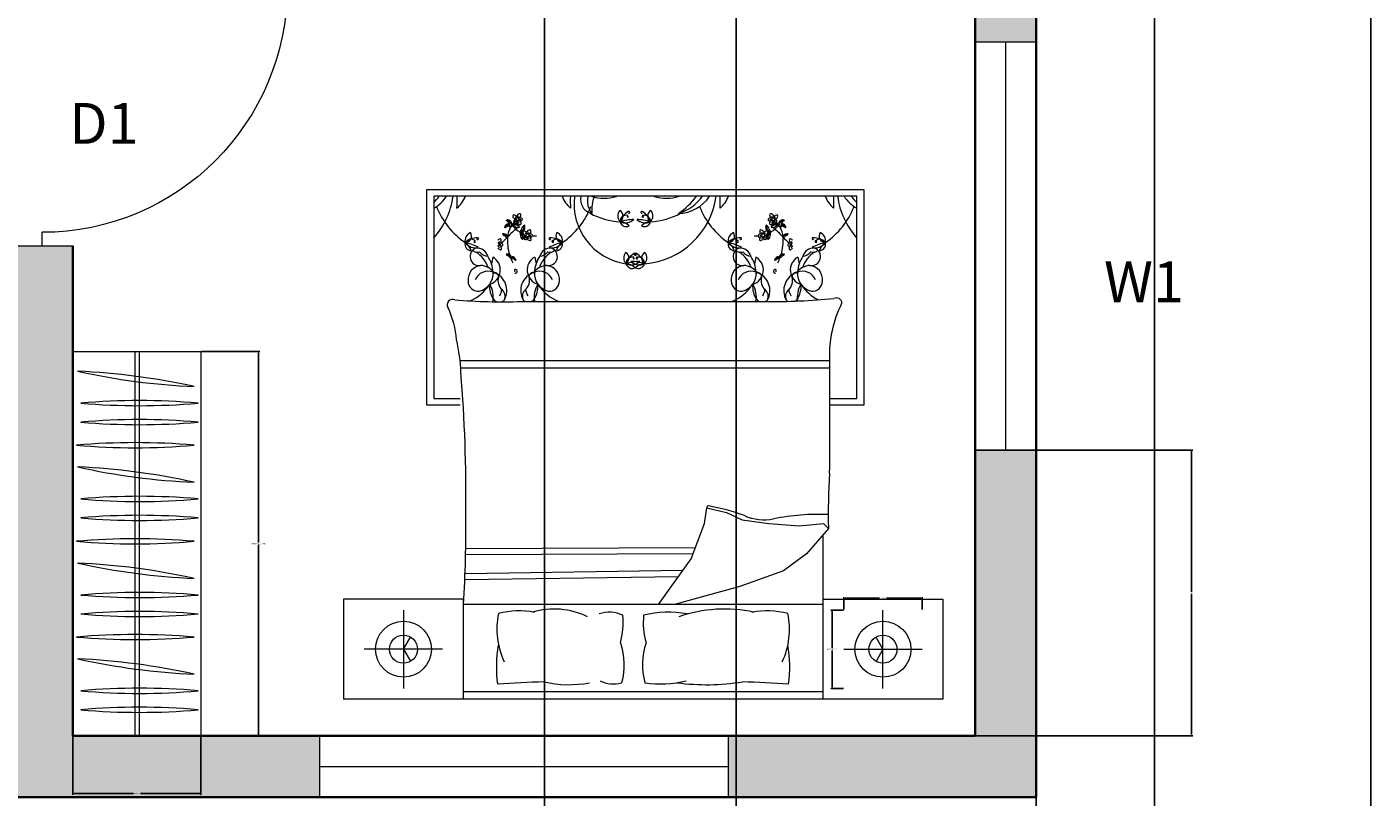
# Model space of a CAD drawing. Units: inches. Extents: x 5 to 421, y -617 to 43.
# Tile 8 of 15: x 223 to 421, y -465 to -351. Entities that reach past the tile are written whole.
import ezdxf

# ---------------------------------------------------------------- set-up
doc = ezdxf.new("R2010")
doc.units = ezdxf.units.IN
doc.header["$MEASUREMENT"] = 0
for name, color, linetype, lineweight in [('A-ANNO-DIMS', 2, 'Continuous', 18), ('A-ANNO-TEXT', 7, 'Continuous', 18), ('A-DOOR', 4, 'Continuous', 20), ('A-FLOR-CASE', 8, 'Continuous', 18), ('A-FURN', 8, 'Continuous', 13), ('A-GLAZ', 4, 'Continuous', 18), ('A-WALL', 7, 'Continuous', 35)]:
    doc.layers.add(name, color=color, linetype=linetype, lineweight=lineweight)
doc.layers.add('A-WALL-PATT', color=251, linetype='Continuous', lineweight=13, true_color=0x636466)
doc.styles.get("Standard").update_dxf_attribs({"font": 'arial.ttf'})
doc.dimstyles.get("Standard").update_dxf_attribs({"dimtxt": 0.18, "dimasz": 0.18, "dimexe": 0.18, "dimexo": 0.0625, "dimgap": 0.09, "dimtad": 0, "dimtih": 1, "dimtoh": 1, "dimdec": 0, "dimzin": 0, "dimdsep": 46, "dimlunit": 3, "dimtxsty": 'Standard', "dimcen": 0.09, "dimadec": 0, "dimazin": 0, "dimtfac": 1, "dimtdec": 0, "dimtofl": 0, "dimtmove": 0, "dimatfit": 3, "dimfxl": 1, "dimtolj": 1, "dimtzin": 0, "dimarcsym": 0})

# ---------------------------------------------------------------- blocks, each defined once
blk = doc.blocks.new('WINDOW-W1-60')
for p, q in [((0, 9), (60, 9)), ((0, 0), (0, 9)), ((60, 9), (60, 0)), ((0, 4.5), (60, 4.5)), ((60, 0), (0, 0))]:
    blk.add_line(p, q)
blk = doc.blocks.new('DOOR-SWING-36')
for p, q in [((35, 0), (35, 36)), ((36, 0), (36, 36))]:
    blk.add_line(p, q)
blk.add_arc((36, 0), 36, 90, 180)
blk = doc.blocks.new('WARDROBE-56')
for p, q in [((0, 56.49), (0, 0)), ((0, 56.49), (18.83, 56.49)), ((9.1, 56.49), (9.1, 0)), ((9.73, 56.49), (9.73, 0)), ((18.83, 56.49), (18.83, 0)), ((0, 0), (18.83, 0))]:
    blk.add_line(p, q)
for centre, start, end in [((22.14, 150.32), 257.508, 267.5023), ((-3.61, -45.4), 77.508, 87.5023), ((9.79, -49.81), 85.0028, 94.9972), ((9.79, 147.6), 265.0028, 274.9972), ((9.79, -52.6), 85.0028, 94.9972), ((9.79, 144.81), 265.0028, 274.9972), ((9.18, -55.99), 85.0028, 94.9972), ((9.18, 141.42), 265.0028, 274.9972), ((22.14, 136.25), 257.508, 267.5023), ((-3.61, -59.47), 77.508, 87.5023), ((9.79, -63.88), 85.0028, 94.9972), ((9.79, 133.52), 265.0028, 274.9972), ((9.79, -66.67), 85.0028, 94.9972), ((9.79, 130.73), 265.0028, 274.9972), ((9.18, -70.11), 85.0028, 94.9972), ((9.18, 127.29), 265.0028, 274.9972), ((-3.61, -73.6), 77.508, 87.5023), ((22.14, 122.12), 257.508, 267.5023), ((9.79, -78.01), 85.0028, 94.9972), ((9.79, 119.4), 265.0028, 274.9972), ((9.79, -80.8), 85.0028, 94.9972), ((9.79, 116.61), 265.0028, 274.9972), ((9.18, -84.19), 85.0028, 94.9972), ((9.18, 113.22), 265.0028, 274.9972), ((-3.61, -87.67), 77.508, 87.5023), ((22.14, 108.05), 257.508, 267.5023), ((9.79, -92.08), 85.0028, 94.9972), ((9.79, 105.32), 265.0028, 274.9972), ((9.79, -94.87), 85.0028, 94.9972), ((9.79, 102.53), 265.0028, 274.9972)]:
    blk.add_arc(centre, 99.08, start, end)
blk = doc.blocks.new('BEDSIDE-LAMP-MASTER')
for p, q in [((5.76, 11.51), (5.76, 0)), ((11.51, 5.76), (0, 5.76))]:
    blk.add_line(p, q)
for points in [[(5.76, 5.76), (6.78, 7.54)], [(5.76, 5.76), (6.78, 3.98)]]:
    blk.add_lwpolyline(points)
for radius in [4.11, 2.06]:
    blk.add_circle((5.76, 5.76), radius)
blk = doc.blocks.new('*D42')
at = {"layer": 'A-ANNO-DIMS', "color": 0, "lineweight": -2, "transparency": 16777216}
for p, q in [((248.31, -399.13), (256.9, -399.13)), ((256.72, -399.31), (256.72, -427.19)), ((256.72, -455.44), (256.72, -427.56)), ((248.31, -455.62), (256.9, -455.62))]:
    blk.add_line(p, q, dxfattribs=at)
at = {"layer": 'A-ANNO-DIMS', "color": 0, "transparency": 16777216}
for points in [[(256.69, -399.31), (256.75, -399.31), (256.72, -399.13)], [(256.69, -455.44), (256.75, -455.44), (256.72, -455.62)]]:
    blk.add_solid(points, dxfattribs=at)
at = {"layer": 'Defpoints', "color": 0, "transparency": 16777216}
for p in [(248.25, -399.13), (256.72, -399.13), (248.25, -455.62)]:
    blk.add_point(p, dxfattribs=at)
at = {"layer": 'A-ANNO-DIMS', "color": 0, "transparency": 16777216, "insert": (256.72, -427.37), "char_height": 0.18, "attachment_point": 5}
blk.add_mtext('\\A1;WARDROBE 56 TYP.', dxfattribs=at)
blk = doc.blocks.new('*D43')
at = {"layer": 'A-ANNO-DIMS', "color": 0, "lineweight": -2, "transparency": 16777216}
for p, q in [((229.42, -455.68), (229.42, -464.27)), ((248.25, -455.68), (248.25, -464.27)), ((229.6, -464.09), (238.31, -464.09)), ((248.07, -464.09), (239.35, -464.09))]:
    blk.add_line(p, q, dxfattribs=at)
at = {"layer": 'A-ANNO-DIMS', "color": 0, "transparency": 16777216}
for points in [[(229.6, -464.06), (229.6, -464.12), (229.42, -464.09)], [(248.07, -464.06), (248.07, -464.12), (248.25, -464.09)]]:
    blk.add_solid(points, dxfattribs=at)
at = {"layer": 'Defpoints', "color": 0, "transparency": 16777216}
for p in [(229.42, -455.62), (248.25, -455.62), (248.25, -464.09)]:
    blk.add_point(p, dxfattribs=at)
at = {"layer": 'A-ANNO-DIMS', "color": 0, "transparency": 16777216, "insert": (238.83, -464.09), "char_height": 0.18, "attachment_point": 5}
blk.add_mtext('\\A1;19 TYP.', dxfattribs=at)
blk = doc.blocks.new('*D52')
at = {"layer": 'A-ANNO-DIMS', "color": 0, "lineweight": -2, "transparency": 16777216}
for p, q in [((342.67, -437.13), (340.83, -437.13)), ((341.01, -437.31), (341.01, -442.71)), ((341.01, -448.46), (341.01, -443.07)), ((342.67, -448.64), (340.83, -448.64))]:
    blk.add_line(p, q, dxfattribs=at)
at = {"layer": 'A-ANNO-DIMS', "color": 0, "transparency": 16777216}
for points in [[(340.98, -437.31), (341.04, -437.31), (341.01, -437.13)], [(340.98, -448.46), (341.04, -448.46), (341.01, -448.64)]]:
    blk.add_solid(points, dxfattribs=at)
at = {"layer": 'Defpoints', "color": 0, "transparency": 16777216}
for p in [(342.74, -437.13), (341.01, -448.64), (342.74, -448.64)]:
    blk.add_point(p, dxfattribs=at)
at = {"layer": 'A-ANNO-DIMS', "color": 0, "transparency": 16777216, "insert": (341.01, -442.89), "char_height": 0.18, "attachment_point": 5}
blk.add_mtext('\\A1;LAMP 12 TYP.', dxfattribs=at)
blk = doc.blocks.new('*D53')
at = {"layer": 'A-ANNO-DIMS', "color": 0, "lineweight": -2, "transparency": 16777216}
for p, q in [((342.74, -437.07), (342.74, -435.22)), ((354.25, -437.07), (354.25, -435.22)), ((342.92, -435.4), (347.97, -435.4)), ((354.07, -435.4), (349.01, -435.4))]:
    blk.add_line(p, q, dxfattribs=at)
at = {"layer": 'A-ANNO-DIMS', "color": 0, "transparency": 16777216}
for points in [[(342.92, -435.37), (342.92, -435.43), (342.74, -435.4)], [(354.07, -435.37), (354.07, -435.43), (354.25, -435.4)]]:
    blk.add_solid(points, dxfattribs=at)
at = {"layer": 'Defpoints', "color": 0, "transparency": 16777216}
for p in [(342.74, -435.4), (342.74, -437.13), (354.25, -437.13)]:
    blk.add_point(p, dxfattribs=at)
at = {"layer": 'A-ANNO-DIMS', "color": 0, "transparency": 16777216, "insert": (348.49, -435.4), "char_height": 0.18, "attachment_point": 5}
blk.add_mtext('\\A1;12 TYP.', dxfattribs=at)
blk = doc.blocks.new('*D55')
at = {"layer": 'A-ANNO-DIMS', "color": 0, "lineweight": -2, "transparency": 16777216}
for p, q in [((370.48, 10.88), (420.4, 10.88)), ((420.22, 10.7), (420.22, -286.69)), ((420.22, -584.44), (420.22, -287.05)), ((169.48, -584.62), (420.4, -584.62))]:
    blk.add_line(p, q, dxfattribs=at)
at = {"layer": 'A-ANNO-DIMS', "color": 0, "transparency": 16777216}
for points in [[(420.19, 10.7), (420.25, 10.7), (420.22, 10.88)], [(420.19, -584.44), (420.25, -584.44), (420.22, -584.62)]]:
    blk.add_solid(points, dxfattribs=at)
at = {"layer": 'Defpoints', "color": 0, "transparency": 16777216}
for p in [(370.42, 10.88), (169.42, -584.62), (420.22, -584.62)]:
    blk.add_point(p, dxfattribs=at)
at = {"layer": 'A-ANNO-DIMS', "color": 0, "transparency": 16777216, "insert": (420.22, -286.87), "char_height": 0.18, "attachment_point": 5}
blk.add_mtext('\\A1;595.5', dxfattribs=at)
blk = doc.blocks.new('*D66')
at = {"layer": 'A-ANNO-DIMS', "color": 0, "lineweight": -2, "transparency": 16777216}
for p, q in [((362.09, -413.62), (394.01, -413.62)), ((393.83, -413.8), (393.83, -434.44)), ((393.83, -455.44), (393.83, -434.8)), ((362.09, -455.62), (394.01, -455.62))]:
    blk.add_line(p, q, dxfattribs=at)
at = {"layer": 'A-ANNO-DIMS', "color": 0, "transparency": 16777216}
for points in [[(393.8, -413.8), (393.86, -413.8), (393.83, -413.62)], [(393.8, -455.44), (393.86, -455.44), (393.83, -455.62)]]:
    blk.add_solid(points, dxfattribs=at)
at = {"layer": 'Defpoints', "color": 0, "transparency": 16777216}
for p in [(362.03, -413.62), (362.03, -455.62), (393.83, -455.62)]:
    blk.add_point(p, dxfattribs=at)
at = {"layer": 'A-ANNO-DIMS', "color": 0, "transparency": 16777216, "insert": (393.83, -434.62), "char_height": 0.18, "attachment_point": 5}
blk.add_mtext('\\A1;42', dxfattribs=at)
blk = doc.blocks.new('*D69')
at = {"layer": 'A-ANNO-DIMS', "color": 0, "lineweight": -2, "transparency": 16777216}
for p, q in [((298.73, -207.41), (298.73, -616.6)), ((326.92, -207.41), (326.92, -616.6)), ((298.91, -616.42), (312.43, -616.42)), ((326.74, -616.42), (313.22, -616.42))]:
    blk.add_line(p, q, dxfattribs=at)
at = {"layer": 'A-ANNO-DIMS', "color": 0, "transparency": 16777216}
for points in [[(298.91, -616.39), (298.91, -616.45), (298.73, -616.42)], [(326.74, -616.39), (326.74, -616.45), (326.92, -616.42)]]:
    blk.add_solid(points, dxfattribs=at)
at = {"layer": 'Defpoints', "color": 0, "transparency": 16777216}
for p in [(298.73, -207.35), (326.92, -207.35), (326.92, -616.42)]:
    blk.add_point(p, dxfattribs=at)
at = {"layer": 'A-ANNO-DIMS', "color": 0, "transparency": 16777216, "insert": (312.82, -616.42), "char_height": 0.18, "attachment_point": 5}
blk.add_mtext('\\A1;28.19', dxfattribs=at)
blk = doc.blocks.new('*D73')
at = {"layer": 'A-ANNO-DIMS', "color": 0, "lineweight": -2, "transparency": 16777216}
for p, q in [((371.03, -247.18), (371.03, -616.6)), ((388.42, -247.18), (388.42, -616.6)), ((371.21, -616.42), (379.27, -616.42)), ((388.24, -616.42), (380.18, -616.42))]:
    blk.add_line(p, q, dxfattribs=at)
at = {"layer": 'A-ANNO-DIMS', "color": 0, "transparency": 16777216}
for points in [[(371.21, -616.39), (371.21, -616.45), (371.03, -616.42)], [(388.24, -616.39), (388.24, -616.45), (388.42, -616.42)]]:
    blk.add_solid(points, dxfattribs=at)
at = {"layer": 'Defpoints', "color": 0, "transparency": 16777216}
for p in [(371.03, -247.12), (388.42, -247.12), (388.42, -616.42)]:
    blk.add_point(p, dxfattribs=at)
at = {"layer": 'A-ANNO-DIMS', "color": 0, "transparency": 16777216, "insert": (379.72, -616.42), "char_height": 0.18, "attachment_point": 5}
blk.add_mtext('\\A1;17.393', dxfattribs=at)

msp = doc.modelspace()

# ---------------------------------------------------------------- hatches: boundary and pattern name
at = {"layer": 'A-WALL-PATT'}
h = msp.add_hatch(color=256, dxfattribs=at)
h.dxf.hatch_style = 1
h.paths.add_polyline_path([(46.4196, -88.1188), (37.4196, -88.1188), (37.4196, -166.6119), (46.4196, -166.6119), (46.4196, -122.6188), (135.4196, -122.6188), (135.4196, -120.3688), (135.4196, -118.1188), (46.4196, -118.1188)])
h.paths.add_polyline_path([(82.4196, 10.8812), (37.4196, 10.8812), (37.4196, -28.1188), (46.4196, -28.1188), (46.4196, 1.8812), (82.4196, 1.8812)])
h.paths.add_polyline_path([(215.5968, 10.8812), (142.4196, 10.8812), (142.4196, 1.8812), (178.4196, 1.8812), (178.4196, -118.1188), (175.4196, -118.1188), (175.4196, -122.6188), (182.9196, -122.6188), (182.9196, -80.6188), (211.9196, -80.6188), (211.9196, -78.3688), (211.9196, -76.1188), (182.9196, -76.1188), (182.9196, 1.8812), (215.5968, 1.8812)])
h.paths.add_polyline_path([(274.4196, 10.8812), (239.5968, 10.8812), (239.5968, 1.8812), (242.9196, 1.8812), (242.9196, -76.1188), (239.9196, -76.1188), (239.9196, -80.6188), (242.9196, -80.6188), (242.9196, -83.6188), (247.4196, -83.6188), (247.4196, 1.8812), (274.4196, 1.8812)])
h.paths.add_polyline_path([(370.4196, 10.8812), (334.4196, 10.8812), (334.4196, 1.8812), (361.4196, 1.8812), (361.4196, -28.1188), (370.4196, -28.1188)])
h.paths.add_polyline_path([(370.4196, -88.1188), (361.4196, -88.1188), (361.4196, -118.1188), (247.4196, -118.1188), (247.4196, -115.1188), (242.9196, -115.1188), (242.9196, -118.1188), (220.4196, -118.1188), (220.4196, -158.6188), (224.9196, -158.6188), (224.9196, -122.6188), (326.9196, -122.6188), (326.9196, -170.7662), (331.4196, -170.7662), (331.4196, -122.6188), (370.4196, -122.6188)])
h.paths.add_polyline_path([(388.4196, -122.6188), (388.4196, -118.1188), (379.4196, -118.1188), (379.4196, -122.6188), (379.4196, -154.8688), (388.4196, -154.8688)])
h.paths.add_polyline_path([(388.4196, -214.8688), (379.4196, -214.8688), (379.4196, -247.1188), (388.4196, -247.1188)])
h.paths.add_polyline_path([(371.0265, -242.6188), (331.4196, -242.6188), (331.4196, -239.6188), (326.9196, -239.6188), (326.9196, -242.6188), (224.9196, -242.6188), (224.9196, -206.6188), (220.4196, -206.6188), (220.4196, -343.6188), (224.9196, -343.6188), (229.4196, -343.6188), (229.4196, -247.1188), (261.5265, -247.1188), (261.5265, -276.1188), (263.7765, -276.1188), (266.0265, -276.1188), (266.0265, -247.1188), (362.0265, -247.1188), (362.0265, -265.1188), (371.0265, -265.1188), (371.0265, -247.1188)])
h.paths.add_polyline_path([(371.0265, -289.1188), (362.0265, -289.1188), (362.0265, -307.1188), (266.0265, -307.1188), (266.0265, -304.1188), (261.5265, -304.1188), (261.5265, -307.1188), (261.5265, -311.6188), (362.0265, -311.6188), (362.0265, -353.6188), (371.0265, -353.6188)])
h.paths.add_polyline_path([(371.0265, -413.6188), (362.0265, -413.6188), (362.0265, -455.6188), (325.7231, -455.6188), (325.7231, -464.6188), (361.4196, -464.6188), (371.0265, -464.6188)])
h.paths.add_polyline_path([(265.7231, -455.6188), (229.4196, -455.6188), (229.4196, -383.6188), (220.4196, -383.6188), (220.4196, -386.6188), (207.4649, -386.6188), (207.4649, -395.6188), (220.4196, -395.6188), (220.4196, -455.6188), (216.0568, -455.6188), (216.0568, -464.6188), (265.7231, -464.6188)])
h.paths.add_polyline_path([(169.4196, -386.6188), (137.9196, -386.6188), (137.9196, -395.6188), (160.4196, -395.6188), (160.4196, -424.2032), (169.4196, -424.2032)])
h.paths.add_polyline_path([(169.4196, -453.7423), (160.4196, -453.7423), (160.4196, -464.6188), (169.4196, -464.6188)])
h.paths.add_polyline_path([(46.4196, -575.6188), (37.4196, -575.6188), (37.4196, -584.6188), (46.4196, -584.6188)])
h.paths.add_polyline_path([(169.4196, -575.6188), (160.4196, -575.6188), (160.4196, -579.5504), (160.4196, -584.6188), (169.4196, -584.6188)])
h.paths.add_polyline_path([(46.4196, -226.6119), (37.4196, -226.6119), (37.4196, -292.8008), (46.4196, -292.8008)])
h.paths.add_polyline_path([(46.4196, -352.8008), (37.4196, -352.8008), (37.4196, -395.6188), (77.9196, -395.6188), (77.9196, -386.6188), (46.4196, -386.6188)])

# ---------------------------------------------------------------- linework, layer by layer
at = {"layer": 'A-DOOR'}
for p, q in [((224.9196, -383.6188), (224.9196, -381.6188)), ((220.4196, -383.6188), (229.4196, -383.6188))]:
    msp.add_line(p, q, dxfattribs=at)
at = {"layer": 'A-FURN'}
for p, q in [((281.441, -375.3025), (345.6729, -375.3025)), ((281.441, -407.0403), (281.441, -375.3025)), ((345.6729, -375.3025), (345.6729, -407.0403)), ((282.4619, -376.3234), (282.4619, -406.0194)), ((344.6519, -376.3234), (282.4619, -376.3234)), ((344.6519, -406.0194), (344.6519, -376.3234)), ((291.1441, -385.2558), (290.9493, -386.2513)), ((297.3016, -385.2558), (297.4964, -386.2513)), ((329.8122, -385.2558), (329.6174, -386.2513)), ((335.9697, -385.2558), (336.1645, -386.2513)), ((295.3636, -391.7921), (331.1354, -391.7921)), ((286.3342, -400.4465), (340.6962, -400.4465)), ((286.4178, -401.5454), (340.696, -401.5454)), ((286.3269, -407.0403), (281.441, -407.0403)), ((282.4619, -406.0194), (286.3455, -406.0194)), ((345.6729, -407.0403), (340.6893, -407.0403)), ((340.6912, -406.0194), (344.6519, -406.0194)), ((322.2678, -424.4143), (322.6247, -422.0959)), ((322.6247, -422.0959), (325.4799, -422.8092)), ((325.4799, -422.8092), (327.7997, -423.8793)), ((320.3049, -429.5861), (322.2678, -424.4143)), ((327.7997, -423.8793), (331.7256, -424.4143)), ((331.7256, -424.4143), (336.1869, -424.7709)), ((336.1869, -424.7709), (339.7559, -424.4143)), ((340.4697, -425.1276), (337.2576, -428.8727)), ((339.7559, -424.4143), (340.4697, -425.1276)), ((339.6809, -450.2295), (339.6809, -426.0473)), ((287.1298, -428.0635), (320.9353, -427.9249)), ((287.1343, -428.9681), (320.5899, -428.8351)), ((337.2576, -428.8727), (333.8671, -431.3694)), ((287.0888, -431.742), (319.0805, -431.2903)), ((315.4769, -436.3064), (320.3049, -429.5861)), ((287.0546, -432.6462), (318.4223, -432.2066)), ((333.8671, -431.3694), (327.4428, -433.6878)), ((327.4428, -433.6878), (317.8355, -436.3064)), ((339.6809, -436.3064), (286.8181, -436.3064)), ((286.8181, -449.0986), (339.6809, -449.0986)), ((357.3018, -450.2295), (269.1972, -450.2295))]:
    msp.add_line(p, q, dxfattribs=at)
for points in [[(286.442, -402.239, 0.05611182), (285.8028, -397.3916, 0.09534134), (284.5645, -392.7225)], [(340.654, -417.0602, 0.00124232), (340.6962, -400.3434, -0.12720156), (342.4625, -392.0121)], [(291.8786, -448.0337, -0.07489676), (291.9855, -442.2789, 0.47281659)], [(309.8999, -441.957, -0.14098958), (310.0762, -447.8279, -0.23524475)], [(313.6623, -441.957, 0.14098958), (313.486, -447.8279, 0.23524475)], [(334.6204, -448.0337, 0.07489676), (334.5136, -442.2789, -0.47281659)]]:
    msp.add_lwpolyline(points, format="xyb", dxfattribs=at)
for points in [[(286.8181, -450.2295), (286.8181, -435.5454), (269.1972, -435.5454), (269.1972, -450.2295)], [(339.6809, -435.5454), (357.3018, -435.5454), (357.3018, -450.2295)]]:
    msp.add_lwpolyline(points, dxfattribs=at)
for centre in [(294.7666, -379.6981), (332.3472, -379.6981), (296.2342, -382.0632), (330.8796, -382.0632)]:
    msp.add_circle(centre, 0.2244, dxfattribs=at)
for centre, radius, start, end in [((279.6683, -373.2323), 5.6062, 299.888429, 326.538275), ((277.6512, -372.1871), 6.9864, 313.518578, 323.696435), ((273.8965, -374.773), 11.5052, 318.114397, 352.255043), ((293.5801, -373.6354), 11.5052, 201.409207, 235.613455), ((282.8082, -374.5291), 4.6779, 311.04544, 337.445257), ((269.9941, -377.0433), 15.9182, 356.348095, 2.591893), ((305.6376, -374.5291), 4.6779, 202.554743, 228.95456), ((294.8657, -373.6354), 11.5052, 304.386545, 338.590793), ((318.4517, -377.0433), 15.9182, 177.408107, 183.651905), ((311.9843, -377.4296), 8.9043, 172.863554, 261.819659), ((306.1077, -376.8094), 2.0651, 166.389819, 259.073851), ((307.6597, -377.093), 2.6114, 162.860876, 221.904868), ((307.5139, -370.2741), 6.3264, 252.979799, 286.456893), ((310.833, -378.2433), 5.1511, 158.117032, 186.619536), ((310.0204, -367.0136), 9.355, 264.364262, 265.621276), ((314.9475, -360.6043), 16.7177, 250.097156, 250.278285), ((312.5646, -374.773), 11.5052, 274.462329, 352.255043), ((316.6631, -370.2741), 6.3264, 253.543107, 287.020201), ((314.1566, -367.0136), 9.355, 274.378724, 275.635738), ((309.2295, -360.6043), 16.7177, 289.721715, 289.902844), ((318.3363, -373.2323), 5.6062, 271.271967, 326.538275), ((312.6477, -370.2229), 10.3922, 304.012338, 324.053042), ((316.3192, -372.1871), 6.9864, 287.850379, 323.696435), ((332.2482, -373.6354), 11.5052, 201.409207, 235.613455), ((308.6622, -377.0433), 15.9182, 356.348095, 2.591893), ((321.4762, -374.5291), 4.6779, 311.04544, 337.445257), ((344.3057, -374.5291), 4.6779, 202.554743, 228.95456), ((333.5337, -373.6354), 11.5052, 304.386545, 338.590793), ((357.1197, -377.0433), 15.9182, 177.408107, 183.651905), ((353.2173, -374.773), 11.5052, 187.744957, 221.885603), ((347.4456, -373.2323), 5.6062, 213.461725, 240.111571), ((349.4627, -372.1871), 6.9864, 216.303565, 226.481422), ((293.3194, -380.0252), 0.2505, 55.607669, 145.646202), ((293.1484, -380.5612), 0.6782, 21.708712, 93.029927), ((289.5734, -385.4013), 6.555, 53.62539, 57.321597), ((293.3564, -380.3932), 0.5841, 342.804199, 79.694321), ((294.2951, -379.277), 0.2223, 134.373191, 211.950101), ((294.7067, -379.0203), 0.7074, 211.950101, 255.244186), ((294.3097, -379.5269), 0.4428, 8.561414, 112.591427), ((294.5189, -380.0102), 0.306, 88.571889, 233.895444), ((294.4343, -379.5089), 0.1486, 352.868017, 97.093987), ((294.278, -379.8321), 0.3088, 298.849254, 359.935492), ((294.3514, -380.0953), 0.3529, 4.212295, 48.15875), ((295.0723, -379.2827), 0.3704, 100.959737, 208.780415), ((295.4722, -379.7761), 0.6812, 132.389629, 156.572429), ((295.1725, -379.8631), 0.3671, 42.320848, 130.211082), ((295.2557, -379.4794), 0.4638, 226.346175, 279.651304), ((294.7764, -380.3389), 0.5396, 7.496845, 71.273729), ((294.7587, -379.0856), 0.5214, 291.638236, 4.946963), ((295.1676, -378.9973), 0.7345, 254.282907, 276.914838), ((295.1067, -379.0555), 0.1721, 4.946963, 127.526288), ((295.301, -379.746), 0.1933, 279.651304, 42.320848), ((310.7315, -368.6106), 11.5052, 242.585402, 265.537671), ((310.7814, -379.2237), 1.2759, 140.885535, 222.212682), ((309.3324, -379.2629), 0.9608, 301.637318, 61.460901), ((310.7769, -380.0441), 0.9412, 76.14802, 182.241514), ((312.589, -381.0242), 2.9097, 121.989022, 161.084052), ((312.2442, -387.761), 8.0487, 92.741826, 107.406963), ((310.5852, -378.4233), 1.8189, 245.689918, 314.458869), ((310.9842, -379.2992), 0.075, 140.190924, 76.020882), ((311.1232, -378.6775), 0.1429, 288.440821, 121.989022), ((311.1465, -378.7473), 0.0694, 171.983321, 288.440821), ((311.9328, -387.761), 8.0487, 72.593037, 87.258174), ((313.5918, -378.4233), 1.8189, 225.541131, 294.310082), ((313.0538, -378.6775), 0.1429, 58.010978, 251.559179), ((313.0305, -378.7473), 0.0694, 251.559179, 8.016679), ((313.2046, -379.2511), 0.1245, 103.85198, 39.924541), ((311.588, -381.0242), 2.9097, 18.915948, 58.010978), ((313.4002, -380.0441), 0.9412, 357.758486, 103.85198), ((314.8446, -379.2629), 0.9608, 118.539099, 238.362682), ((313.3956, -379.2237), 1.2759, 317.787318, 39.114465), ((313.4455, -368.6106), 11.5052, 274.462329, 297.414598), ((331.8128, -379.746), 0.1933, 137.679152, 260.348696), ((331.9413, -379.8631), 0.3671, 49.788918, 137.679152), ((331.8581, -379.4794), 0.4638, 260.348696, 313.653825), ((332.3374, -380.3389), 0.5396, 108.726271, 172.503155), ((332.3551, -379.0856), 0.5214, 175.053037, 248.361764), ((332.0071, -379.0555), 0.1721, 52.473712, 175.053037), ((331.9462, -378.9973), 0.7345, 263.085162, 285.717093), ((331.6417, -379.7761), 0.6812, 23.427571, 47.610371), ((332.0416, -379.2827), 0.3704, 331.219585, 79.040263), ((332.8041, -379.5269), 0.4428, 67.408573, 171.438586), ((332.7624, -380.0953), 0.3529, 131.84125, 175.787705), ((332.8358, -379.8321), 0.3088, 180.064508, 241.150746), ((332.6795, -379.5089), 0.1486, 82.906013, 187.131983), ((332.4072, -379.0203), 0.7074, 284.755814, 328.049899), ((332.595, -380.0102), 0.306, 306.104556, 91.428111), ((332.8188, -379.277), 0.2223, 328.049899, 45.626809), ((333.7575, -380.3932), 0.5841, 100.305679, 197.195801), ((333.9654, -380.5612), 0.6782, 86.970073, 158.291288), ((333.7945, -380.0252), 0.2505, 34.353798, 124.392331), ((337.5405, -385.4013), 6.555, 122.678403, 126.37461), ((288.3289, -382.8585), 1.2759, 110.961322, 192.288469), ((287.0536, -382.1696), 0.9608, 271.713105, 31.536686), ((292.633, -384.3393), 2.4847, 82.869762, 91.673614), ((292.9779, -381.6563), 0.4626, 205.53786, 258.674386), ((292.3125, -383.2259), 1.3925, 59.344007, 79.741218), ((293.134, -380.8449), 0.2505, 123.097874, 213.136405), ((293.5636, -381.208), 0.6782, 92.31716, 160.520132), ((296.6663, -386.3636), 6.555, 121.115593, 124.811802), ((293.4881, -380.9516), 0.5841, 82.600826, 147.184524), ((293.413, -380.9738), 0.2594, 45.735421, 121.115593), ((296.9474, -382.6271), 3.6582, 150.795916, 175.243979), ((302.2139, -390.4166), 12.0383, 127.825561, 137.758756), ((293.307, -380.3324), 0.2594, 338.245218, 53.62539), ((293.7297, -380.501), 0.1957, 158.245218, 340.639457), ((293.7306, -380.6479), 0.1957, 225.735421, 48.129663), ((297.4093, -378.8648), 3.9079, 201.708712, 206.218055), ((294.2992, -381.5343), 1.0227, 40.936473, 112.769517), ((293.9616, -381.1904), 0.6019, 49.381187, 95.545644), ((294.4021, -380.9514), 0.6217, 61.183768, 141.679176), ((296.9474, -382.6271), 3.6582, 137.508292, 145.996664), ((297.3237, -377.7682), 4.3882, 220.182023, 239.455983), ((294.4848, -380.0933), 0.2198, 228.29465, 6.247442), ((294.8245, -380.1843), 0.7235, 229.381187, 289.995928), ((294.3563, -381.0646), 0.7431, 15.64837, 62.295742), ((295.0769, -380.0457), 0.3742, 183.634966, 258.436272), ((295.0281, -379.9105), 0.2143, 178.132531, 268.891946), ((295.1437, -380.3127), 0.1734, 215.075197, 14.764439), ((295.0627, -382.1683), 0.6217, 3.877392, 87.150123), ((294.7822, -380.5808), 1.0227, 287.888952, 359.721997), ((294.7502, -381.0617), 0.6019, 305.112828, 351.277285), ((294.6236, -381.9267), 0.6019, 352.074807, 38.239267), ((294.5166, -382.3966), 1.0227, 343.630094, 55.463139), ((295.2401, -380.956), 0.6217, 271.4625, 339.4747), ((296.0602, -381.2627), 0.7235, 110.662543, 171.277285), ((295.7627, -381.6421), 0.2223, 134.373191, 211.950101), ((297.3237, -377.7682), 4.3882, 246.152261, 246.949926), ((296.1743, -381.3854), 0.7074, 211.950101, 255.244186), ((295.7773, -381.892), 0.4428, 8.561414, 112.591427), ((295.1315, -380.9), 0.7431, 338.362726, 25.010099), ((295.9019, -381.874), 0.1486, 352.868017, 97.093987), ((296.5399, -381.6477), 0.3704, 100.959737, 208.780415), ((296.9398, -382.1412), 0.6812, 132.389629, 156.572429), ((296.6401, -382.2281), 0.3671, 42.320848, 130.211082), ((296.2263, -381.4507), 0.5214, 291.638236, 4.946963), ((296.5743, -381.4206), 0.1721, 4.946963, 127.526288), ((301.3922, -382.1696), 0.9608, 148.463314, 268.286895), ((300.1169, -382.8585), 1.2759, 347.711531, 69.038678), ((309.7864, -382.0454), 1.9651, 44.627337, 88.541544), ((310.7523, -379.8149), 0.9538, 196.196251, 296.972629), ((314.3906, -382.0454), 1.9651, 91.458456, 135.372663), ((313.4247, -379.8149), 0.9538, 243.027371, 343.803749), ((326.997, -382.8585), 1.2759, 110.961322, 192.288469), ((325.7216, -382.1696), 0.9608, 271.713105, 31.536686), ((330.4737, -382.2281), 0.3671, 49.788918, 137.679152), ((330.8875, -381.4507), 0.5214, 175.053037, 248.361764), ((330.5395, -381.4206), 0.1721, 52.473712, 175.053037), ((330.1741, -382.1412), 0.6812, 23.427571, 47.610371), ((330.574, -381.6477), 0.3704, 331.219585, 79.040263), ((331.3365, -381.892), 0.4428, 67.408573, 171.438586), ((331.2119, -381.874), 0.1486, 82.906013, 187.131983), ((330.9396, -381.3854), 0.7074, 284.755814, 328.049899), ((331.9823, -380.9), 0.7431, 154.989901, 201.637274), ((331.8738, -380.956), 0.6217, 200.5253, 268.5375), ((332.3316, -380.5808), 1.0227, 180.278003, 252.111048), ((331.0536, -381.2627), 0.7235, 8.722715, 69.337457), ((332.0511, -382.1683), 0.6217, 92.849877, 176.122608), ((331.3512, -381.6421), 0.2223, 328.049899, 45.626809), ((329.7902, -377.7682), 4.3882, 293.050074, 293.847739), ((332.5973, -382.3966), 1.0227, 124.536861, 196.369906), ((332.3637, -381.0617), 0.6019, 188.722715, 234.887172), ((331.9701, -380.3127), 0.1734, 165.235561, 324.924803), ((332.4902, -381.9267), 0.6019, 141.760733, 187.925193), ((329.7902, -377.7682), 4.3882, 300.544017, 319.817977), ((332.7575, -381.0646), 0.7431, 117.704258, 164.35163), ((332.8146, -381.5343), 1.0227, 67.230483, 139.063527), ((332.2894, -380.1843), 0.7235, 250.004072, 310.618813), ((332.0857, -379.9105), 0.2143, 271.108054, 1.867469), ((332.037, -380.0457), 0.3742, 281.563728, 356.365034), ((324.8999, -390.4166), 12.0383, 42.241244, 52.174439), ((332.629, -380.0933), 0.2198, 173.752558, 311.70535), ((332.7117, -380.9514), 0.6217, 38.320824, 118.816232), ((333.1522, -381.1904), 0.6019, 84.454356, 130.618813), ((330.1665, -382.6271), 3.6582, 34.003336, 42.491708), ((333.3832, -380.6479), 0.1957, 131.870337, 314.264579), ((333.3841, -380.501), 0.1957, 199.360543, 21.754782), ((329.7045, -378.8648), 3.9079, 333.781945, 338.291288), ((330.1665, -382.6271), 3.6582, 4.756021, 29.204084), ((333.7008, -380.9738), 0.2594, 58.884407, 134.264579), ((333.8068, -380.3324), 0.2594, 126.37461, 201.754782), ((333.6257, -380.9516), 0.5841, 32.815476, 97.399174), ((333.5502, -381.208), 0.6782, 19.479868, 87.68284), ((330.4475, -386.3636), 6.555, 55.188198, 58.884407), ((334.8014, -383.2259), 1.3925, 100.258782, 120.655993), ((333.9798, -380.8449), 0.2505, 326.863595, 56.902126), ((334.4808, -384.3393), 2.4847, 88.326386, 97.130238), ((334.136, -381.6563), 0.4626, 281.325614, 334.46214), ((340.0603, -382.1696), 0.9608, 148.463314, 268.286895), ((338.7849, -382.8585), 1.2759, 347.711531, 69.038678), ((288.0088, -383.3564), 0.9538, 166.272036, 267.048413), ((288.9973, -385.3207), 2.9097, 92.064805, 131.159835), ((287.9157, -383.5673), 0.9412, 46.223807, 152.317301), ((285.3379, -390.9874), 8.0487, 62.81761, 77.482743), ((288.5582, -382.0669), 1.8189, 215.765707, 284.534651), ((286.0589, -384.8077), 1.9651, 14.703123, 58.617328), ((288.4671, -383.0251), 0.075, 110.266709, 46.227077), ((288.883, -382.6277), 0.0694, 142.059106, 258.516605), ((288.8977, -382.5557), 0.1429, 258.516605, 92.064805), ((292.1901, -382.9811), 0.3704, 100.959737, 142.237914), ((291.8845, -383.3966), 0.2244, 273.276835, 86.723165), ((292.146, -383.6089), 0.2143, 178.132531, 268.891946), ((292.5901, -383.4746), 0.6812, 132.389629, 156.572429), ((292.2904, -383.5615), 0.3671, 42.320848, 130.211082), ((292.3736, -383.1779), 0.4638, 226.346175, 279.651304), ((291.8943, -384.0374), 0.5396, 7.496845, 71.273729), ((291.8766, -382.7841), 0.5214, 291.638236, 4.946963), ((292.2855, -382.6958), 0.7345, 254.282907, 276.914838), ((292.2246, -382.754), 0.1721, 4.946963, 127.526288), ((287.1991, -376.6022), 8.3653, 307.954095, 316.845875), ((292.4189, -383.4445), 0.1933, 279.651304, 42.320848), ((292.0114, -383.2221), 1.4155, 43.692881, 51.789879), ((292.8801, -382.2922), 0.4228, 355.713146, 81.656778), ((292.646, -382.6632), 0.7384, 27.365857, 59.344007), ((293.2008, -382.1754), 0.1795, 202.558349, 304.234253), ((300.5827, -382.811), 7.2972, 176.172317, 196.415821), ((295.9364, -382.1094), 0.7235, 172.074807, 232.689549), ((294.9426, -382.1909), 0.7431, 318.34199, 4.989364), ((295.9865, -382.3753), 0.306, 88.571889, 233.895444), ((295.9524, -382.4584), 0.2198, 228.29465, 6.247442), ((295.7456, -382.1971), 0.3088, 298.849254, 359.935492), ((295.819, -382.4604), 0.3529, 4.212295, 48.15875), ((296.5445, -382.4107), 0.3742, 183.634966, 258.436272), ((296.4957, -382.2755), 0.2143, 178.132531, 268.891946), ((296.7233, -381.8444), 0.4638, 226.346175, 279.651304), ((296.244, -382.704), 0.5396, 7.496845, 71.273729), ((296.6352, -381.3624), 0.7345, 254.282907, 276.914838), ((296.6113, -382.6777), 0.1734, 215.075197, 14.764439), ((296.7686, -382.1111), 0.1933, 279.651304, 42.320848), ((297.3237, -377.7682), 4.3882, 265.241474, 272.892907), ((299.5481, -382.5557), 0.1429, 87.935195, 281.483395), ((299.8876, -382.0669), 1.8189, 255.465349, 324.234293), ((303.1079, -390.9874), 8.0487, 102.517257, 117.18239), ((299.4484, -385.3207), 2.9097, 48.840165, 87.935195), ((299.5628, -382.6277), 0.0694, 281.483395, 37.940894), ((299.965, -382.9776), 0.1245, 133.776193, 69.718346), ((300.53, -383.5673), 0.9412, 27.682699, 133.776193), ((300.437, -383.3564), 0.9538, 272.951587, 13.727964), ((302.3868, -384.8077), 1.9651, 121.382672, 165.296877), ((326.6769, -383.3564), 0.9538, 166.272036, 267.048413), ((327.6654, -385.3207), 2.9097, 92.064805, 131.159835), ((326.5838, -383.5673), 0.9412, 46.223807, 152.317301), ((324.727, -384.8077), 1.9651, 14.703123, 58.617328), ((327.2263, -382.0669), 1.8189, 215.765707, 284.534651), ((324.0059, -390.9874), 8.0487, 62.81761, 77.482743), ((327.1351, -383.0251), 0.075, 110.266709, 46.227077), ((327.5511, -382.6277), 0.0694, 142.059106, 258.516605), ((327.5657, -382.5557), 0.1429, 258.516605, 92.064805), ((329.7902, -377.7682), 4.3882, 267.107093, 274.758526), ((330.3452, -382.1111), 0.1933, 137.679152, 260.348696), ((330.3905, -381.8444), 0.4638, 260.348696, 313.653825), ((330.5025, -382.6777), 0.1734, 165.235561, 324.924803), ((330.8698, -382.704), 0.5396, 108.726271, 172.503155), ((330.4786, -381.3624), 0.7345, 263.085162, 285.717093), ((330.6181, -382.2755), 0.2143, 271.108054, 1.867469), ((330.5694, -382.4107), 0.3742, 281.563728, 356.365034), ((331.1614, -382.4584), 0.2198, 173.752558, 311.70535), ((331.2948, -382.4604), 0.3529, 131.84125, 175.787705), ((331.3682, -382.1971), 0.3088, 180.064508, 241.150746), ((331.1274, -382.3753), 0.306, 306.104556, 91.428111), ((332.1712, -382.1909), 0.7431, 175.010636, 221.65801), ((331.1775, -382.1094), 0.7235, 307.310451, 7.925193), ((326.5311, -382.811), 7.2972, 343.584179, 3.827683), ((334.2337, -382.2922), 0.4228, 98.343222, 184.286854), ((334.4678, -382.6632), 0.7384, 120.655993, 152.634143), ((333.9131, -382.1754), 0.1795, 235.765747, 337.441651), ((339.9147, -376.6022), 8.3653, 223.154125, 232.045905), ((335.1024, -383.2221), 1.4155, 128.210121, 136.307119), ((334.6949, -383.4445), 0.1933, 137.679152, 260.348696), ((334.8234, -383.5615), 0.3671, 49.788918, 137.679152), ((334.7402, -383.1779), 0.4638, 260.348696, 313.653825), ((335.2195, -384.0374), 0.5396, 108.726271, 172.503155), ((335.2372, -382.7841), 0.5214, 175.053037, 248.361764), ((334.8893, -382.754), 0.1721, 52.473712, 175.053037), ((334.8283, -382.6958), 0.7345, 263.085162, 285.717093), ((334.9679, -383.6089), 0.2143, 271.108054, 1.867469), ((334.5238, -383.4746), 0.6812, 23.427571, 47.610371), ((334.9237, -382.9811), 0.3704, 37.762086, 79.040263), ((335.2294, -383.3966), 0.2244, 93.276835, 266.723165), ((338.2162, -382.5557), 0.1429, 87.935195, 281.483395), ((341.776, -390.9874), 8.0487, 102.517257, 117.18239), ((338.5556, -382.0669), 1.8189, 255.465349, 324.234293), ((338.1165, -385.3207), 2.9097, 48.840165, 87.935195), ((338.2308, -382.6277), 0.0694, 281.483395, 37.940894), ((338.6331, -382.9776), 0.1245, 133.776193, 69.718346), ((339.1981, -383.5673), 0.9412, 27.682699, 133.776193), ((341.0549, -384.8077), 1.9651, 121.382672, 165.296877), ((339.105, -383.3564), 0.9538, 272.951587, 13.727964), ((289.1289, -385.1842), 1.3222, 109.131157, 279.736024), ((288.8567, -383.7515), 0.8104, 216.731946, 296.024452), ((286.5073, -388.0947), 4.1595, 18.295495, 58.738626), ((288.8117, -385.5821), 1.6512, 15.695503, 94.030982), ((290.5902, -383.387), 1.7586, 218.417454, 263.833797), ((286.4683, -387.7595), 4.728, 3.492404, 33.711716), ((290.052, -387.1544), 2.1903, 286.866299, 60.091459), ((292.1947, -383.7442), 0.3742, 217.364203, 258.436272), ((292.2616, -384.0112), 0.1734, 215.075197, 14.764439), ((293.1579, -387.3039), 2.4847, 82.869762, 91.673614), ((293.5028, -384.6208), 0.4626, 205.53786, 258.674386), ((292.8374, -386.1905), 1.3925, 59.344007, 79.741218), ((292.5363, -386.1867), 1.4155, 43.692881, 51.789879), ((293.405, -385.2568), 0.4228, 355.713146, 81.656778), ((293.1709, -385.6278), 0.7384, 27.365857, 59.344007), ((293.7257, -385.14), 0.1795, 202.558349, 304.234253), ((300.5827, -382.811), 7.2972, 200.105922, 206.996805), ((294.0052, -385.3073), 0.1795, 173.945725, 275.621623), ((294.0536, -385.6451), 0.4228, 36.523195, 122.466832), ((293.8371, -386.0267), 0.7384, 58.835967, 90.814121), ((293.6442, -386.85), 1.4155, 66.390094, 74.487092), ((294.568, -385.2586), 0.4626, 219.505588, 272.642118), ((293.4986, -386.5864), 1.3925, 38.438755, 58.835967), ((292.3659, -386.8296), 2.4847, 26.506361, 35.310211), ((298.3938, -387.1544), 2.1903, 119.908541, 253.133701), ((301.9774, -387.7595), 4.728, 146.288284, 176.507596), ((301.9385, -388.0947), 4.1595, 121.261374, 161.704505), ((299.6341, -385.5821), 1.6512, 85.969018, 164.304497), ((297.8556, -383.387), 1.7586, 276.166203, 321.582546), ((299.3168, -385.1842), 1.3222, 260.263976, 70.868843), ((299.589, -383.7515), 0.8104, 243.975548, 323.268054), ((311.6623, -385.3861), 1.2759, 140.885535, 222.212682), ((310.2133, -385.4252), 0.9608, 301.637318, 61.460901), ((311.6577, -386.2065), 0.9412, 76.14802, 182.241514), ((313.4699, -387.1866), 2.9097, 121.989022, 161.084052), ((311.8651, -385.4615), 0.075, 140.190924, 76.020882), ((312.0041, -384.8399), 0.1429, 288.440821, 121.989022), ((312.0274, -384.9096), 0.0694, 171.983321, 288.440821), ((312.1729, -384.8399), 0.1429, 58.010978, 251.559179), ((312.1496, -384.9096), 0.0694, 251.559179, 8.016679), ((312.3237, -385.4135), 0.1245, 103.85198, 39.924541), ((310.7072, -387.1866), 2.9097, 18.915948, 58.010978), ((312.5193, -386.2065), 0.9412, 357.758486, 103.85198), ((313.9637, -385.4252), 0.9608, 118.539099, 238.362682), ((312.5147, -385.3861), 1.2759, 317.787318, 39.114465), ((327.797, -385.1842), 1.3222, 109.131157, 279.736024), ((327.5248, -383.7515), 0.8104, 216.731946, 296.024452), ((325.1754, -388.0947), 4.1595, 18.295495, 58.738626), ((327.4797, -385.5821), 1.6512, 15.695503, 94.030982), ((329.2582, -383.387), 1.7586, 218.417454, 263.833797), ((325.1364, -387.7595), 4.728, 3.492404, 33.711716), ((328.7201, -387.1544), 2.1903, 286.866299, 60.091459), ((334.748, -386.8296), 2.4847, 144.689789, 153.493639), ((333.6152, -386.5864), 1.3925, 121.164033, 141.561245), ((332.5458, -385.2586), 0.4626, 267.357882, 320.494412), ((333.0602, -385.6451), 0.4228, 57.533168, 143.476805), ((333.2767, -386.0267), 0.7384, 89.185879, 121.164033), ((333.4697, -386.85), 1.4155, 105.512908, 113.609906), ((326.5311, -382.811), 7.2972, 333.003195, 339.894078), ((333.1086, -385.3073), 0.1795, 264.378377, 6.054275), ((333.7088, -385.2568), 0.4228, 98.343222, 184.286854), ((333.9429, -385.6278), 0.7384, 120.655993, 152.634143), ((333.3882, -385.14), 0.1795, 235.765747, 337.441651), ((334.5775, -386.1867), 1.4155, 128.210121, 136.307119), ((334.2765, -386.1905), 1.3925, 100.258782, 120.655993), ((333.9559, -387.3039), 2.4847, 88.326386, 97.130238), ((333.6111, -384.6208), 0.4626, 281.325614, 334.46214), ((334.8522, -384.0112), 0.1734, 165.235561, 324.924803), ((337.0618, -387.1544), 2.1903, 119.908541, 253.133701), ((334.9191, -383.7442), 0.3742, 281.563728, 322.635797), ((340.6455, -387.7595), 4.728, 146.288284, 176.507596), ((340.6065, -388.0947), 4.1595, 121.261374, 161.704505), ((338.3022, -385.5821), 1.6512, 85.969018, 164.304497), ((336.5237, -383.387), 1.7586, 276.166203, 321.582546), ((337.9849, -385.1842), 1.3222, 260.263976, 70.868843), ((338.2571, -383.7515), 0.8104, 243.975548, 323.268054), ((289.6133, -388.5766), 2.1054, 97.114253, 185.055148), ((290.4408, -389.3749), 2.0446, 68.577852, 158.418133), ((288.5466, -387.6889), 2.6499, 283.079005, 4.706656), ((289.2472, -389.0445), 2.5593, 35.959859, 87.640897), ((294.0556, -389.5553), 3.3979, 143.65552, 147.29887), ((291.4389, -388.0751), 0.5468, 344.852873, 102.695942), ((290.3916, -390.1918), 2.8077, 330.8249, 70.717823), ((294.4757, -387.2456), 0.1698, 79.561551, 257.29493), ((294.4565, -387.3501), 0.2761, 259.586441, 79.561551), ((298.0542, -390.1918), 2.8077, 109.282177, 209.1751), ((297.0068, -388.0751), 0.5468, 77.304058, 195.147127), ((299.1986, -389.0445), 2.5593, 92.359103, 144.040141), ((294.3902, -389.5553), 3.3979, 32.70113, 36.34448), ((299.8992, -387.6889), 2.6499, 175.293344, 256.920995), ((298.005, -389.3749), 2.0446, 21.581867, 111.422148), ((298.8325, -388.5766), 2.1054, 354.944852, 82.885747), ((311.4661, -384.5856), 1.8189, 245.689918, 314.458869), ((313.1251, -393.9234), 8.0487, 92.741826, 107.406963), ((311.6332, -385.9773), 0.9538, 196.196251, 296.972629), ((310.6673, -388.2078), 1.9651, 44.627337, 88.541544), ((312.7109, -384.5856), 1.8189, 225.541131, 294.310082), ((311.0519, -393.9234), 8.0487, 72.593037, 87.258174), ((312.5438, -385.9773), 0.9538, 243.027371, 343.803749), ((313.5097, -388.2078), 1.9651, 91.458456, 135.372663), ((328.2814, -388.5766), 2.1054, 97.114253, 185.055148), ((329.1089, -389.3749), 2.0446, 68.577852, 158.418133), ((327.2147, -387.6889), 2.6499, 283.079005, 4.706656), ((327.9153, -389.0445), 2.5593, 35.959859, 87.640897), ((332.7237, -389.5553), 3.3979, 143.65552, 147.29887), ((330.107, -388.0751), 0.5468, 344.852873, 102.695942), ((329.0597, -390.1918), 2.8077, 330.8249, 70.717823), ((332.6574, -387.3501), 0.2761, 100.438449, 280.413559), ((332.6381, -387.2456), 0.1698, 282.70507, 100.438449), ((336.7222, -390.1918), 2.8077, 109.282177, 209.1751), ((335.6749, -388.0751), 0.5468, 77.304058, 195.147127), ((337.8666, -389.0445), 2.5593, 92.359103, 144.040141), ((333.0582, -389.5553), 3.3979, 32.70113, 36.34448), ((338.5672, -387.6889), 2.6499, 175.293344, 256.920995), ((336.673, -389.3749), 2.0446, 21.581867, 111.422148), ((337.5005, -388.5766), 2.1054, 354.944852, 82.885747), ((289.0033, -388.7895), 1.4875, 178.94622, 275.514429), ((285.1188, -385.5876), 6.6682, 293.645326, 326.332878), ((294.0556, -389.5553), 3.3979, 175.269627, 214.214953), ((287.5645, -391.1402), 3.6502, 349.248989, 31.178216), ((293.7103, -388.69), 1.8062, 164.852873, 228.434694), ((294.7355, -388.69), 1.8062, 311.565306, 15.147127), ((294.3902, -389.5553), 3.3979, 325.785047, 4.730373), ((300.8813, -391.1402), 3.6502, 148.821784, 190.286655), ((303.327, -385.5876), 6.6682, 213.667122, 248.505868), ((299.4425, -388.7895), 1.4875, 264.485571, 1.05378), ((327.6714, -388.7895), 1.4875, 178.94622, 275.514429), ((323.7869, -385.5876), 6.6682, 291.494132, 326.332878), ((332.7237, -389.5553), 3.3979, 175.269627, 214.214953), ((326.2326, -391.1402), 3.6502, 349.713345, 31.178216), ((332.3783, -388.69), 1.8062, 164.852873, 228.434694), ((333.4036, -388.69), 1.8062, 311.565306, 15.147127), ((333.0582, -389.5553), 3.3979, 325.785047, 4.730373), ((339.5493, -391.1402), 3.6502, 148.821784, 189.155424), ((341.995, -385.5876), 6.6682, 213.667122, 243.299656), ((338.1105, -388.7895), 1.4875, 264.485571, 1.05378), ((285.2316, -392.2755), 0.8031, 66.521858, 213.826416), ((292.6654, -306.102), 85.7326, 265.240242, 271.803508), ((292.0856, -390.8174), 1.0611, 217.675028, 252.581425), ((289.9677, -389.6838), 2.5326, 330.085135, 352.564012), ((292.0856, -390.8174), 1.0611, 286.634335, 315.548308), ((291.6372, -391.0278), 1.3183, 336.164593, 48.434694), ((296.8086, -391.0278), 1.3183, 131.565306, 203.835407), ((296.3601, -390.8174), 1.0611, 224.451692, 246.714357), ((298.478, -389.6838), 2.5326, 187.435988, 209.914865), ((296.3601, -390.8174), 1.0611, 293.285643, 322.324972), ((330.7537, -390.8174), 1.0611, 217.675028, 246.714357), ((328.6358, -389.6838), 2.5326, 330.085135, 352.564012), ((332.1867, -300.0802), 91.7179, 269.343254, 275.688691), ((330.7537, -390.8174), 1.0611, 293.229008, 315.548308), ((330.3053, -391.0278), 1.3183, 336.164593, 48.434694), ((335.4766, -391.0278), 1.3183, 131.565306, 203.835407), ((335.0282, -390.8174), 1.0611, 224.451692, 243.558008), ((337.1461, -389.6838), 2.5326, 187.435988, 209.914865), ((335.0282, -390.8174), 1.0611, 300.029301, 322.324972), ((341.6515, -392.0685), 0.8129, 3.979981, 117.341241), ((80.6815, -419.7831), 206.5071, 359.114536, 4.873507), ((421.2525, -422.9374), 80.8125, 175.829411, 181.553045), ((128.8753, -425.5389), 158.3095, 356.099968, 0.928176), ((322.8248, -422.024), 0.2126, 88.862345, 199.753635), ((316.5076, -455.3894), 34.1678, 70.119422, 79.33829), ((331.0139, -416.6928), 7.1719, 246.261584, 281.339199), ((338.9619, -456.3275), 33.2519, 87.45188, 101.339199), ((295.0214, -449.0648), 11.8071, 78.963113, 104.896067), ((300.1173, -448.1948), 11.2153, 63.876108, 106.174639), ((325.2621, -457.4573), 20.4785, 78.039745, 109.261524), ((331.4776, -449.0648), 11.8071, 75.103933, 101.036887), ((303.1033, -439.9685), 11.3553, 168.241659, 204.8684), ((308.2779, -442.12), 4.6706, 65.01826, 108.540728), ((299.5141, -439.0123), 10.7952, 344.170723, 5.987112), ((324.0481, -439.0123), 10.7952, 174.012888, 195.829277), ((316.9714, -452.9861), 15.5369, 79.861689, 103.623756), ((323.3958, -439.9685), 11.3553, 335.1316, 11.758341), ((340.4414, -1286.4987), 839.8702, 92.8502247, 93.3147907), ((302.3355, -432.6173), 15.4881, 256.342714, 281.1841), ((308.8673, -443.6404), 4.3585, 243.343742, 286.102557), ((315.7998, -432.3002), 15.6992, 261.524927, 283.959959), ((322.5483, -416.1521), 31.9533, 262.219583, 279.496983), ((286.0577, -1286.4987), 839.8702, 86.6852093, 87.1497753)]:
    msp.add_arc(centre, radius, start, end, dxfattribs=at)
at = {"layer": 'A-WALL'}
for p, q in [((371.0265, -247.1188), (371.0265, -464.6188)), ((362.0265, -311.6188), (362.0265, -455.6188)), ((229.4196, -383.6188), (229.4196, -455.6188)), ((229.4196, -455.6188), (362.0265, -455.6188)), ((207.4649, -464.6188), (361.4196, -464.6188)), ((371.0265, -464.6188), (361.4196, -464.6188))]:
    msp.add_line(p, q, dxfattribs=at)

# ---------------------------------------------------------------- block references
at = {"layer": 'A-DOOR', "extrusion": (0, 0, -1), "zscale": -1, "rotation": 90.00000000000006}
msp.add_blockref('DOOR-SWING-36', (-224.9196, -381.6188), dxfattribs=at)
at = {"layer": 'A-FLOR-CASE'}
msp.add_blockref('WARDROBE-56', (229.4196, -455.6188), dxfattribs=at)
at = {"layer": 'A-FURN'}
msp.add_blockref('BEDSIDE-LAMP-MASTER', (272.2515, -448.6436), dxfattribs=at)
at = {"layer": 'A-FURN', "rotation": 180}
msp.add_blockref('BEDSIDE-LAMP-MASTER', (354.2475, -437.1313), dxfattribs=at)
at = {"layer": 'A-GLAZ', "rotation": 89.99999999999976}
msp.add_blockref('WINDOW-W1-60', (371.0265, -413.6188), dxfattribs=at)
at = {"layer": 'A-GLAZ'}
msp.add_blockref('WINDOW-W1-60', (265.7231, -464.6188), dxfattribs=at)

# ---------------------------------------------------------------- texts
at = {"layer": 'A-ANNO-TEXT', "char_height": 6, "attachment_point": 1}
for s, insert in [('D1', (228.8969, -362.6102)), ('W1', (380.9837, -385.9054))]:
    msp.add_mtext(s, dxfattribs=dict(at, insert=insert))

# ---------------------------------------------------------------- dimensions: what is measured, and where the dimension line sits
at = {"layer": 'A-ANNO-DIMS'}
for base, p1, p2, angle, override, picture, middle in [((420.2196, -584.6188), (370.4196, 10.8812), (169.4196, -584.6188), 90, {"dimdec": 1, "dimlfac": 1, "dimrnd": 0, "dimzin": 0, "dimdsep": 46, "dimlunit": 2}, '*D55', (420.2196, -286.8688)), ((393.8265, -455.6188), (362.0265, -413.6188), (362.0265, -455.6188), 270, {"dimdec": 0, "dimlfac": 1, "dimrnd": 0, "dimzin": 0, "dimdsep": 46, "dimlunit": 2}, '*D66', (393.8265, -434.6188))]:
    dim = msp.add_linear_dim(base=base, p1=p1, p2=p2, angle=angle, dimstyle='Standard', override=override, dxfattribs=at)
    dim.commit()
    dim.dimension.update_dxf_attribs({"geometry": picture, "text_midpoint": middle})
for base, p1, p2, override, picture, middle in [((326.9196, -616.4188), (298.7283, -207.3464), (326.9196, -207.3464), {"dimdec": 2, "dimlfac": 1, "dimrnd": 0, "dimzin": 0, "dimdsep": 46, "dimlunit": 2}, '*D69', (312.8239, -616.4188)), ((388.4196, -616.4188), (371.0265, -247.1188), (388.4196, -247.1188), {"dimdec": 3, "dimlfac": 1, "dimrnd": 0, "dimzin": 0, "dimdsep": 46, "dimlunit": 2}, '*D73', (379.7231, -616.4188))]:
    dim = msp.add_linear_dim(base=base, p1=p1, p2=p2, dimstyle='Standard', override=override, dxfattribs=at)
    dim.commit()
    dim.dimension.update_dxf_attribs({"geometry": picture, "text_midpoint": middle})
for base, p1, p2, angle, text, picture, middle in [((256.7231, -399.1287), (248.2496, -455.6188), (248.2496, -399.1287), 90, 'WARDROBE <> TYP.', '*D42', (256.7231, -427.3738)), ((342.7352, -435.4044), (354.2475, -437.1313), (342.7352, -437.1313), 180, '<> TYP.', '*D53', (348.4914, -435.4044)), ((341.0083, -448.6436), (342.7352, -437.1313), (342.7352, -448.6436), 270, 'LAMP <> TYP.', '*D52', (341.0083, -442.8874))]:
    dim = msp.add_linear_dim(base=base, p1=p1, p2=p2, angle=angle, text=text, dimstyle='Standard', override={"dimdec": 0, "dimlfac": 1, "dimrnd": 0, "dimzin": 0, "dimdsep": 46, "dimlunit": 2}, dxfattribs=at)
    dim.commit()
    dim.dimension.update_dxf_attribs({"geometry": picture, "text_midpoint": middle})
dim = msp.add_linear_dim(base=(248.2496, -464.0923), p1=(229.4196, -455.6188), p2=(248.2496, -455.6188), text='<> TYP.', dimstyle='Standard', override={"dimdec": 0, "dimlfac": 1, "dimrnd": 0, "dimzin": 0, "dimdsep": 46, "dimlunit": 2}, dxfattribs=at)
dim.commit()
dim.dimension.update_dxf_attribs({"geometry": '*D43', "text_midpoint": (238.8346, -464.0923)})

doc.saveas('drawing.dxf')
